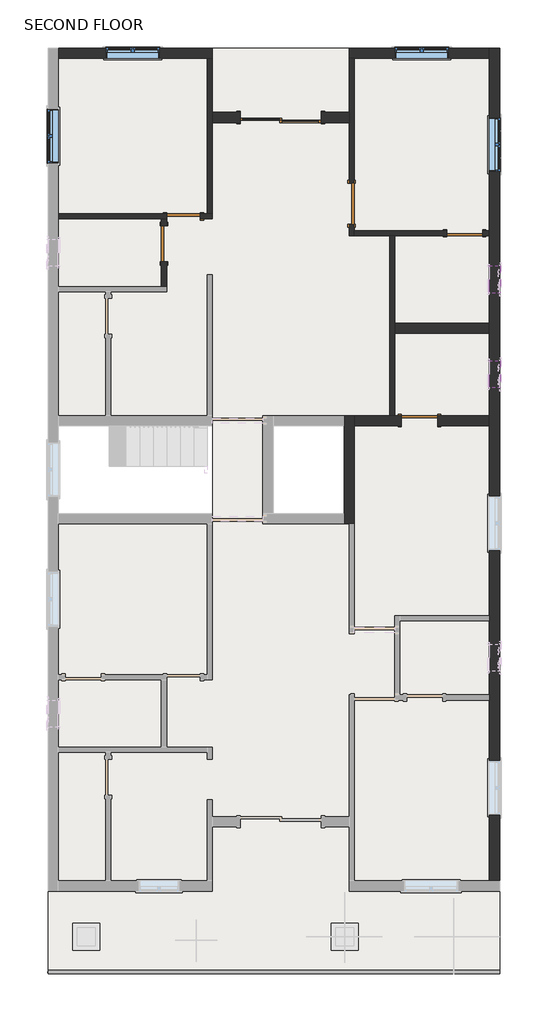
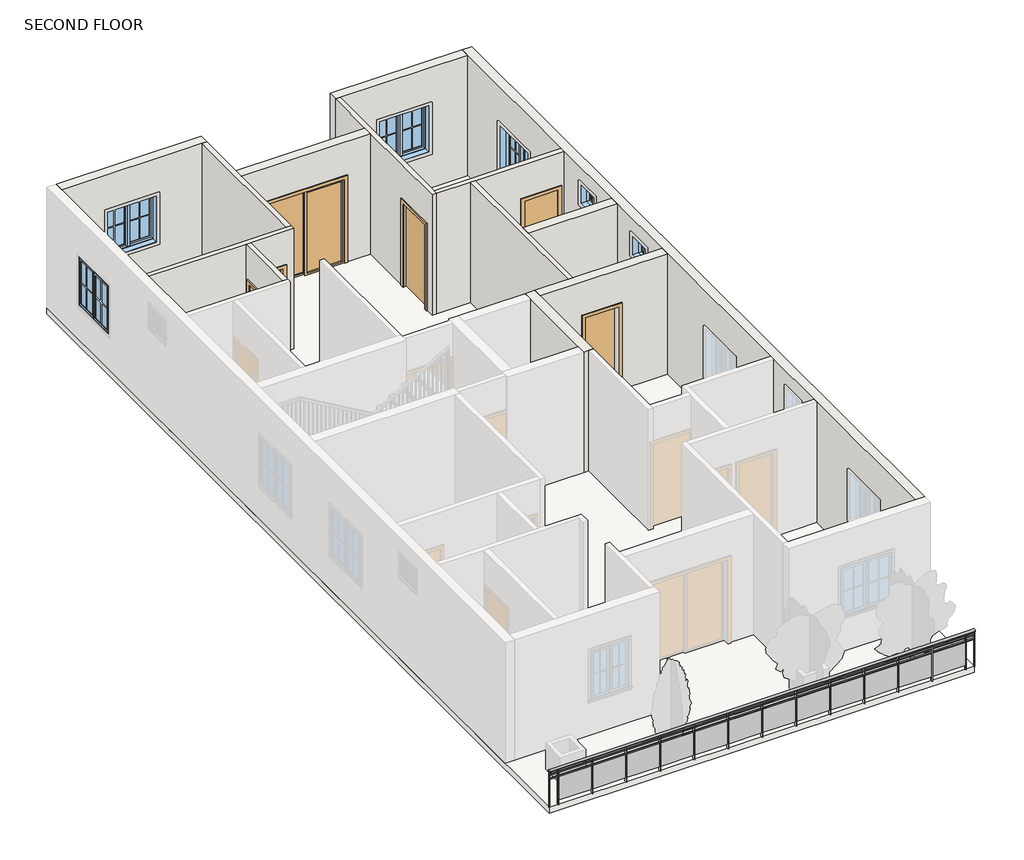
# One storey, part 2 of 4: 13 walls, 6 doors, 6 windows, 1 railing, 1 slab.
"""IFC4 building model written with IfcOpenShell, lengths in millimetres."""

from ifc_helpers import new_model, si_unit, point, frame, origin, place, context, project, spatial, polyline, ellipse_curve, trimmed, outline, extrude, faceted_brep, transform, mapped, element, save
from ifc_brep_helpers import plane_surface, extruded_surface, advanced_brep
from components import door_d4d75d1e, door_214872d5, door_d141acb4, door_38851409, door_7b345704, single_flush_3_x7_e5f9f3c4, window_79894727, window_casement_double_4_x4_af3140d2

model = new_model("IFC4")

# Units and contexts
model_context = context("Model", 3, world=origin())
ifc_project = project(units=[si_unit("LENGTHUNIT", "METRE", prefix="MILLI")], contexts=[model_context])

# Site, building, storey
site = spatial("IfcSite", under=ifc_project)
building = spatial("IfcBuilding", under=site)
storey = spatial("IfcBuildingStorey", under=building, Name="SECOND FLOOR", Elevation=6400.8)

# Doors
placement = place(None, origin())
door_shape = door_d4d75d1e(model_context)
element("IfcDoor", 1, ObjectType="Door-Double-Sliding : 72\" x 84\"", at=placement, inside=storey, context=model_context, shape_type="MappedRepresentation", body=[
    mapped(door_shape, transform((-1119.4789041, 8623.7153263, 6400.8), x_axis=(-1.0, 0.0, 0.0), y_axis=(0.0, -1.0, 0.0), z_axis=(0.0, 0.0, 1.0))),
])
door_2_shape = door_214872d5(model_context)
element("IfcDoor", 2, ObjectType="Single-Flush : 2'6\"X7'", at=placement, inside=storey, context=model_context, shape_type="MappedRepresentation", body=[
    mapped(door_2_shape, transform((-3310.2289041, 6267.8653263, 6400.8), x_axis=(1.0, 0.0, 0.0), y_axis=(0.0, 1.0, 0.0), z_axis=(0.0, 0.0, 1.0))),
])
door_3_shape = door_d141acb4(model_context)
element("IfcDoor", 3, ObjectType="Single-Flush : 2'8\"X7'", at=placement, inside=storey, context=model_context, shape_type="MappedRepresentation", body=[
    mapped(door_3_shape, transform((-3748.3789041, 5651.9153263, 6400.8), x_axis=(0.0, 1.0, 0.0), y_axis=(-1.0, 0.0, 0.0), z_axis=(0.0, 0.0, 1.0))),
])
door_4_shape = door_38851409(model_context)
element("IfcDoor", 4, ObjectType="Single-Flush : 2'8\"X7'", at=placement, inside=storey, context=model_context, shape_type="MappedRepresentation", body=[
    mapped(door_4_shape, transform((3027.0710959, 5886.8653263, 6400.8), x_axis=(1.0, 0.0, 0.0), y_axis=(0.0, 1.0, 0.0), z_axis=(0.0, 0.0, 1.0))),
])
door_5_shape = door_7b345704(model_context)
element("IfcDoor", 5, ObjectType="Single-Flush : 2'8\"X7'", at=placement, inside=storey, context=model_context, shape_type="MappedRepresentation", body=[
    mapped(door_5_shape, transform((2011.0710959, 1664.1153263, 6400.8), x_axis=(-1.0, 0.0, 0.0), y_axis=(0.0, -1.0, 0.0), z_axis=(0.0, 0.0, 1.0))),
])
single_flush_3_x7_shape = single_flush_3_x7_e5f9f3c4(model_context)
element("IfcDoor", 6, ObjectType="Single-Flush : 3'X7'", at=placement, inside=storey, context=model_context, shape_type="MappedRepresentation", body=[
    mapped(single_flush_3_x7_shape, transform((480.7210959, 6553.6153263, 6400.8), x_axis=(0.0, -1.0, 0.0), y_axis=(1.0, 0.0, 0.0), z_axis=(0.0, 0.0, 1.0))),
])

# Railing
element("IfcRailing", 7, ObjectType="Glass Panel - Bottom Fill", at=placement, inside=storey, context=model_context, shape_type="SolidModel", body=[
    advanced_brep(
    [(-6358.2289041, -10731.0846737, 7315.2), (-6358.2289041, -10807.2846737, 7315.2), (3814.4710959, -10731.0846737, 7315.2), (3814.4710959, -10807.2846737, 7315.2)],
    [
        (0, 1, ellipse_curve(frame((-6358.2289041, -10769.1846737, 7315.2), z_axis=(-1.0, 0.0, 0.0), x_axis=(0.0, -1.0, 0.0)), 38.1, 28.575)),
        (1, 0, ellipse_curve(frame((-6358.2289041, -10769.1846737, 7315.2), z_axis=(-1.0, 0.0, 0.0), x_axis=(0.0, -1.0, 0.0)), 38.1, 28.575)),
        (2, 3, ellipse_curve(frame((3814.4710959, -10769.1846737, 7315.2), z_axis=(1.0, 0.0, 0.0), x_axis=(0.0, -1.0, 0.0)), 38.1, 28.575)),
        (3, 2, ellipse_curve(frame((3814.4710959, -10769.1846737, 7315.2), z_axis=(1.0, 0.0, 0.0), x_axis=(0.0, -1.0, 0.0)), 38.1, 28.575)),
        (0, 2),
        (3, 1),
    ],
    [
        plane_surface(frame((-6358.2289041, -10769.1846737, 7315.2), z_axis=(-1.0, 0.0, 0.0), x_axis=(0.0, 1.0, 0.0))),
        plane_surface(frame((3814.4710959, -10769.1846737, 7315.2), z_axis=(1.0, 0.0, 0.0), x_axis=(0.0, 1.0, 0.0))),
        extruded_surface(trimmed(ellipse_curve(frame((3814.4710959, -10769.1846737, 7315.2), z_axis=(-1.0, 0.0, 0.0), x_axis=(0.0, -1.0, 0.0)), 38.1, 28.575), [point((3814.4710959, -10731.0846737, 7315.2))], [point((3814.4710959, -10807.2846737, 7315.2))], True, "CARTESIAN"), (-10172.7, 0.0, 0.0), 10172.7),
        extruded_surface(trimmed(ellipse_curve(frame((3814.4710959, -10769.1846737, 7315.2), z_axis=(-1.0, 0.0, 0.0), x_axis=(0.0, -1.0, 0.0)), 38.1, 28.575), [point((3814.4710959, -10807.2846737, 7315.2))], [point((3814.4710959, -10731.0846737, 7315.2))], True, "CARTESIAN"), (-10172.7, 0.0, 0.0), 10172.7),
    ],
    [
        (0, [[1, 2]]),
        (1, [[3, 4]]),
        (2, [[-1, 5, -4, 6]]),
        (3, [[-2, -6, -3, -5]]),
    ],
),
    extrude(outline(polyline([(-6358.2289041, -10781.8846737), (-6358.2289041, -10756.4846737), (3814.4710959, -10756.4846737), (3814.4710959, -10781.8846737), (-6358.2289041, -10781.8846737)])), frame((0.0, 0.0, 7200.9), z_axis=(0.0, 0.0, 1.0), x_axis=(1.0, 0.0, 0.0)), (0.0, 0.0, 1.0), 25.4),
    extrude(outline(polyline([(-6358.2289041, -10781.8846737), (-6358.2289041, -10756.4846737), (3814.4710959, -10756.4846737), (3814.4710959, -10781.8846737), (-6358.2289041, -10781.8846737)])), frame((0.0, 0.0, 7099.3), z_axis=(0.0, 0.0, 1.0), x_axis=(1.0, 0.0, 0.0)), (0.0, 0.0, 1.0), 25.4),
    extrude(outline(polyline([(3598.5710959, -10794.5846737), (3598.5710959, -10743.7846737), (3611.2710959, -10743.7846737), (3611.2710959, -10794.5846737), (3598.5710959, -10794.5846737)])), frame((0.0, 0.0, 6400.8), z_axis=(0.0, 0.0, 1.0), x_axis=(1.0, 0.0, 0.0)), (0.0, 0.0, 1.0), 885.825),
    extrude(outline(polyline([(2792.1210959, -10762.6495167), (3604.9210959, -10762.6495167), (3604.9210959, -10768.9995167), (2792.1210959, -10768.9995167), (2792.1210959, -10762.6495167)])), frame((0.0, 0.0, 6502.4), z_axis=(0.0, 0.0, 1.0), x_axis=(1.0, 0.0, 0.0)), (0.0, 0.0, 1.0), 596.9),
    extrude(outline(polyline([(2785.7710959, -10794.5846737), (2785.7710959, -10743.7846737), (2798.4710959, -10743.7846737), (2798.4710959, -10794.5846737), (2785.7710959, -10794.5846737)])), frame((0.0, 0.0, 6400.8), z_axis=(0.0, 0.0, 1.0), x_axis=(1.0, 0.0, 0.0)), (0.0, 0.0, 1.0), 885.825),
    extrude(outline(polyline([(1979.3210959, -10762.6495167), (2792.1210959, -10762.6495167), (2792.1210959, -10768.9995167), (1979.3210959, -10768.9995167), (1979.3210959, -10762.6495167)])), frame((0.0, 0.0, 6502.4), z_axis=(0.0, 0.0, 1.0), x_axis=(1.0, 0.0, 0.0)), (0.0, 0.0, 1.0), 596.9),
    extrude(outline(polyline([(1972.9710959, -10794.5846737), (1972.9710959, -10743.7846737), (1985.6710959, -10743.7846737), (1985.6710959, -10794.5846737), (1972.9710959, -10794.5846737)])), frame((0.0, 0.0, 6400.8), z_axis=(0.0, 0.0, 1.0), x_axis=(1.0, 0.0, 0.0)), (0.0, 0.0, 1.0), 885.825),
    extrude(outline(polyline([(1166.5210959, -10762.6495167), (1979.3210959, -10762.6495167), (1979.3210959, -10768.9995167), (1166.5210959, -10768.9995167), (1166.5210959, -10762.6495167)])), frame((0.0, 0.0, 6502.4), z_axis=(0.0, 0.0, 1.0), x_axis=(1.0, 0.0, 0.0)), (0.0, 0.0, 1.0), 596.9),
    extrude(outline(polyline([(1160.1710959, -10794.5846737), (1160.1710959, -10743.7846737), (1172.8710959, -10743.7846737), (1172.8710959, -10794.5846737), (1160.1710959, -10794.5846737)])), frame((0.0, 0.0, 6400.8), z_axis=(0.0, 0.0, 1.0), x_axis=(1.0, 0.0, 0.0)), (0.0, 0.0, 1.0), 885.825),
    extrude(outline(polyline([(353.7210959, -10762.6495167), (1166.5210959, -10762.6495167), (1166.5210959, -10768.9995167), (353.7210959, -10768.9995167), (353.7210959, -10762.6495167)])), frame((0.0, 0.0, 6502.4), z_axis=(0.0, 0.0, 1.0), x_axis=(1.0, 0.0, 0.0)), (0.0, 0.0, 1.0), 596.9),
    extrude(outline(polyline([(347.3710959, -10794.5846737), (347.3710959, -10743.7846737), (360.0710959, -10743.7846737), (360.0710959, -10794.5846737), (347.3710959, -10794.5846737)])), frame((0.0, 0.0, 6400.8), z_axis=(0.0, 0.0, 1.0), x_axis=(1.0, 0.0, 0.0)), (0.0, 0.0, 1.0), 885.825),
    extrude(outline(polyline([(-459.0789041, -10762.6495167), (353.7210959, -10762.6495167), (353.7210959, -10768.9995167), (-459.0789041, -10768.9995167), (-459.0789041, -10762.6495167)])), frame((0.0, 0.0, 6502.4), z_axis=(0.0, 0.0, 1.0), x_axis=(1.0, 0.0, 0.0)), (0.0, 0.0, 1.0), 596.9),
    extrude(outline(polyline([(-465.4289041, -10794.5846737), (-465.4289041, -10743.7846737), (-452.7289041, -10743.7846737), (-452.7289041, -10794.5846737), (-465.4289041, -10794.5846737)])), frame((0.0, 0.0, 6400.8), z_axis=(0.0, 0.0, 1.0), x_axis=(1.0, 0.0, 0.0)), (0.0, 0.0, 1.0), 885.825),
    extrude(outline(polyline([(-1271.8789041, -10762.6495167), (-459.0789041, -10762.6495167), (-459.0789041, -10768.9995167), (-1271.8789041, -10768.9995167), (-1271.8789041, -10762.6495167)])), frame((0.0, 0.0, 6502.4), z_axis=(0.0, 0.0, 1.0), x_axis=(1.0, 0.0, 0.0)), (0.0, 0.0, 1.0), 596.9),
    extrude(outline(polyline([(-1278.2289041, -10794.5846737), (-1278.2289041, -10743.7846737), (-1265.5289041, -10743.7846737), (-1265.5289041, -10794.5846737), (-1278.2289041, -10794.5846737)])), frame((0.0, 0.0, 6400.8), z_axis=(0.0, 0.0, 1.0), x_axis=(1.0, 0.0, 0.0)), (0.0, 0.0, 1.0), 885.825),
    extrude(outline(polyline([(-2084.6789041, -10762.6495167), (-1271.8789041, -10762.6495167), (-1271.8789041, -10768.9995167), (-2084.6789041, -10768.9995167), (-2084.6789041, -10762.6495167)])), frame((0.0, 0.0, 6502.4), z_axis=(0.0, 0.0, 1.0), x_axis=(1.0, 0.0, 0.0)), (0.0, 0.0, 1.0), 596.9),
    extrude(outline(polyline([(-2091.0289041, -10794.5846737), (-2091.0289041, -10743.7846737), (-2078.3289041, -10743.7846737), (-2078.3289041, -10794.5846737), (-2091.0289041, -10794.5846737)])), frame((0.0, 0.0, 6400.8), z_axis=(0.0, 0.0, 1.0), x_axis=(1.0, 0.0, 0.0)), (0.0, 0.0, 1.0), 885.825),
    extrude(outline(polyline([(-2897.4789041, -10762.6495167), (-2084.6789041, -10762.6495167), (-2084.6789041, -10768.9995167), (-2897.4789041, -10768.9995167), (-2897.4789041, -10762.6495167)])), frame((0.0, 0.0, 6502.4), z_axis=(0.0, 0.0, 1.0), x_axis=(1.0, 0.0, 0.0)), (0.0, 0.0, 1.0), 596.9),
    extrude(outline(polyline([(-2903.8289041, -10794.5846737), (-2903.8289041, -10743.7846737), (-2891.1289041, -10743.7846737), (-2891.1289041, -10794.5846737), (-2903.8289041, -10794.5846737)])), frame((0.0, 0.0, 6400.8), z_axis=(0.0, 0.0, 1.0), x_axis=(1.0, 0.0, 0.0)), (0.0, 0.0, 1.0), 885.825),
    extrude(outline(polyline([(-3710.2789041, -10762.6495167), (-2897.4789041, -10762.6495167), (-2897.4789041, -10768.9995167), (-3710.2789041, -10768.9995167), (-3710.2789041, -10762.6495167)])), frame((0.0, 0.0, 6502.4), z_axis=(0.0, 0.0, 1.0), x_axis=(1.0, 0.0, 0.0)), (0.0, 0.0, 1.0), 596.9),
    extrude(outline(polyline([(-3716.6289041, -10794.5846737), (-3716.6289041, -10743.7846737), (-3703.9289041, -10743.7846737), (-3703.9289041, -10794.5846737), (-3716.6289041, -10794.5846737)])), frame((0.0, 0.0, 6400.8), z_axis=(0.0, 0.0, 1.0), x_axis=(1.0, 0.0, 0.0)), (0.0, 0.0, 1.0), 885.825),
    extrude(outline(polyline([(-4523.0789041, -10762.6495167), (-3710.2789041, -10762.6495167), (-3710.2789041, -10768.9995167), (-4523.0789041, -10768.9995167), (-4523.0789041, -10762.6495167)])), frame((0.0, 0.0, 6502.4), z_axis=(0.0, 0.0, 1.0), x_axis=(1.0, 0.0, 0.0)), (0.0, 0.0, 1.0), 596.9),
    extrude(outline(polyline([(-4529.4289041, -10794.5846737), (-4529.4289041, -10743.7846737), (-4516.7289041, -10743.7846737), (-4516.7289041, -10794.5846737), (-4529.4289041, -10794.5846737)])), frame((0.0, 0.0, 6400.8), z_axis=(0.0, 0.0, 1.0), x_axis=(1.0, 0.0, 0.0)), (0.0, 0.0, 1.0), 885.825),
    extrude(outline(polyline([(-5335.8789041, -10762.6495167), (-4523.0789041, -10762.6495167), (-4523.0789041, -10768.9995167), (-5335.8789041, -10768.9995167), (-5335.8789041, -10762.6495167)])), frame((0.0, 0.0, 6502.4), z_axis=(0.0, 0.0, 1.0), x_axis=(1.0, 0.0, 0.0)), (0.0, 0.0, 1.0), 596.9),
    extrude(outline(polyline([(-5342.2289041, -10794.5846737), (-5342.2289041, -10743.7846737), (-5329.5289041, -10743.7846737), (-5329.5289041, -10794.5846737), (-5342.2289041, -10794.5846737)])), frame((0.0, 0.0, 6400.8), z_axis=(0.0, 0.0, 1.0), x_axis=(1.0, 0.0, 0.0)), (0.0, 0.0, 1.0), 885.825),
    extrude(outline(polyline([(-6148.6789041, -10762.6495167), (-5335.8789041, -10762.6495167), (-5335.8789041, -10768.9995167), (-6148.6789041, -10768.9995167), (-6148.6789041, -10762.6495167)])), frame((0.0, 0.0, 6502.4), z_axis=(0.0, 0.0, 1.0), x_axis=(1.0, 0.0, 0.0)), (0.0, 0.0, 1.0), 596.9),
    extrude(outline(polyline([(-6155.0289041, -10794.5846737), (-6155.0289041, -10743.7846737), (-6142.3289041, -10743.7846737), (-6142.3289041, -10794.5846737), (-6155.0289041, -10794.5846737)])), frame((0.0, 0.0, 6400.8), z_axis=(0.0, 0.0, 1.0), x_axis=(1.0, 0.0, 0.0)), (0.0, 0.0, 1.0), 885.825),
    extrude(outline(polyline([(3801.7710959, -10778.7096737), (3801.7710959, -10759.6596737), (3820.8210959, -10759.6596737), (3820.8210959, -10778.7096737), (3801.7710959, -10778.7096737)])), frame((0.0, 0.0, 6400.8), z_axis=(0.0, 0.0, 1.0), x_axis=(1.0, 0.0, 0.0)), (0.0, 0.0, 1.0), 885.825),
    extrude(outline(polyline([(-6364.5789041, -10778.7096737), (-6364.5789041, -10759.6596737), (-6345.5289041, -10759.6596737), (-6345.5289041, -10778.7096737), (-6364.5789041, -10778.7096737)])), frame((0.0, 0.0, 6400.8), z_axis=(0.0, 0.0, 1.0), x_axis=(1.0, 0.0, 0.0)), (0.0, 0.0, 1.0), 885.825),
])

# Slab
element("IfcSlab", 8, ObjectType="6\"", at=placement, inside=storey, context=model_context, shape_type="SweptSolid", body=[
    extrude(outline(polyline([(3814.4710959, 10058.8153263), (3814.4710959, -10769.1846737), (-6358.2289041, -10769.1846737), (-6358.2289041, 10058.8153263), (3814.4710959, 10058.8153263)]), holes=[polyline([(-2662.5289041, 1549.8153263), (-6129.6289041, 1549.8153263), (-6129.6289041, -431.3846737), (-2662.5289041, -431.3846737), (-2662.5289041, 1549.8153263)]), polyline([(537.8710959, 1778.4153263), (-1519.5289041, 1778.4153263), (-1519.5289041, -659.9846737), (537.8710959, -659.9846737), (537.8710959, 1778.4153263)])]), frame((0.0, 0.0, 6248.4), z_axis=(0.0, 0.0, 1.0), x_axis=(1.0, 0.0, 0.0)), (0.0, 0.0, 1.0), 152.4),
])

# Walls
element("IfcWall", 9, ObjectType="4.5\"", at=placement, inside=storey, context=model_context, shape_type="SweptSolid", body=[
    extrude(outline(polyline([(6210.7153263, 6400.8), (6058.3153263, 6400.8), (6058.3153263, 8534.4), (5245.5153263, 8534.4), (5245.5153263, 6400.8), (4686.7153263, 6400.8), (4686.7153263, 9448.8), (6210.7153263, 9448.8), (6210.7153263, 6400.8)])), frame((-3805.5289041, 0.0, 0.0), z_axis=(1.0, 0.0, 0.0), x_axis=(0.0, 1.0, 0.0)), (0.0, 0.0, 1.0), 114.3),
])
element("IfcWall", 10, ObjectType="4.5\"", at=placement, inside=storey, context=model_context, shape_type="Brep", body=[
    faceted_brep([(-2929.2289041, 6210.7153263, 8534.4), (-2929.2289041, 6210.7153263, 6400.8), (-2662.5289041, 6210.7153263, 6400.8), (-2662.5289041, 6210.7153263, 9448.8), (-3691.2289041, 6210.7153263, 9448.8), (-3805.5289041, 6210.7153263, 9448.8), (-6129.6289041, 6210.7153263, 9448.8), (-6129.6289041, 6210.7153263, 6400.8), (-3805.5289041, 6210.7153263, 6400.8), (-3691.2289041, 6210.7153263, 6400.8), (-3691.2289041, 6210.7153263, 8534.4), (-2662.5289041, 6325.0153263, 6400.8), (-2776.8289041, 6325.0153263, 6400.8), (-2929.2289041, 6325.0153263, 6400.8), (-2929.2289041, 6325.0153263, 8534.4), (-3691.2289041, 6325.0153263, 8534.4), (-3691.2289041, 6325.0153263, 6400.8), (-6129.6289041, 6325.0153263, 6400.8), (-6129.6289041, 6325.0153263, 9448.8), (-2776.8289041, 6325.0153263, 9448.8), (-2662.5289041, 6325.0153263, 9448.8)], [[[0, 1, 2, 3, 4, 5, 6, 7, 8, 9, 10]], [[11, 12, 13, 14, 15, 16, 17, 18, 19, 20]], [[2, 1, 13, 12, 11]], [[9, 8, 7, 17, 16]], [[6, 5, 4, 3, 20, 19, 18]], [[7, 6, 18, 17]], [[3, 2, 11, 20]], [[14, 13, 1, 0]], [[15, 14, 0, 10]], [[16, 15, 10, 9]]]),
])
element("IfcWall", 11, ObjectType="4.5\"", at=placement, inside=storey, context=model_context, shape_type="Brep", body=[
    faceted_brep([(-2662.5289041, 6325.0153263, 6400.8), (-2662.5289041, 8382.4153263, 6400.8), (-2662.5289041, 8611.0153263, 6400.8), (-2662.5289041, 9830.2153263, 6400.8), (-2662.5289041, 9830.2153263, 9448.8), (-2662.5289041, 8611.0153263, 9448.8), (-2662.5289041, 8382.4153263, 9448.8), (-2662.5289041, 6325.0153263, 9448.8), (-2776.8289041, 6325.0153263, 6400.8), (-2776.8289041, 6325.0153263, 9448.8), (-2776.8289041, 9830.2153263, 9448.8), (-2776.8289041, 9830.2153263, 6400.8)], [[[0, 1, 2, 3, 4, 5, 6, 7]], [[8, 9, 10, 11]], [[3, 2, 1, 0, 8, 11]], [[7, 6, 5, 4, 10, 9]], [[0, 7, 9, 8]], [[4, 3, 11, 10]]]),
])
element("IfcWall", 12, ObjectType="4.5\"", at=placement, inside=storey, context=model_context, shape_type="Brep", body=[
    faceted_brep([(423.5710959, 6096.4153263, 8534.4), (423.5710959, 6096.4153263, 6400.8), (423.5710959, 5829.7153263, 6400.8), (423.5710959, 5829.7153263, 9448.8), (423.5710959, 8382.4153263, 9448.8), (423.5710959, 8611.0153263, 9448.8), (423.5710959, 9830.2153263, 9448.8), (423.5710959, 9830.2153263, 6400.8), (423.5710959, 8611.0153263, 6400.8), (423.5710959, 8382.4153263, 6400.8), (423.5710959, 7010.8153263, 6400.8), (423.5710959, 7010.8153263, 8534.4), (537.8710959, 5829.7153263, 6400.8), (537.8710959, 5944.0153263, 6400.8), (537.8710959, 6096.4153263, 6400.8), (537.8710959, 6096.4153263, 8534.4), (537.8710959, 7010.8153263, 8534.4), (537.8710959, 7010.8153263, 6400.8), (537.8710959, 9830.2153263, 6400.8), (537.8710959, 9830.2153263, 9448.8), (537.8710959, 5944.0153263, 9448.8), (537.8710959, 5829.7153263, 9448.8)], [[[0, 1, 2, 3, 4, 5, 6, 7, 8, 9, 10, 11]], [[12, 13, 14, 15, 16, 17, 18, 19, 20, 21]], [[2, 1, 14, 13, 12]], [[10, 9, 8, 7, 18, 17]], [[6, 5, 4, 3, 21, 20, 19]], [[7, 6, 19, 18]], [[3, 2, 12, 21]], [[15, 14, 1, 0]], [[16, 15, 0, 11]], [[17, 16, 11, 10]]]),
])
element("IfcWall", 13, ObjectType="4.5\"", at=placement, inside=storey, context=model_context, shape_type="Brep", body=[
    faceted_brep([(3433.4710959, 5829.7153263, 8534.4), (3433.4710959, 5829.7153263, 6400.8), (3585.8710959, 5829.7153263, 6400.8), (3585.8710959, 5829.7153263, 9448.8), (1452.2710959, 5829.7153263, 9448.8), (1337.9710959, 5829.7153263, 9448.8), (537.8710959, 5829.7153263, 9448.8), (537.8710959, 5829.7153263, 6400.8), (1337.9710959, 5829.7153263, 6400.8), (1452.2710959, 5829.7153263, 6400.8), (2620.6710959, 5829.7153263, 6400.8), (2620.6710959, 5829.7153263, 8534.4), (3585.8710959, 5944.0153263, 6400.8), (3433.4710959, 5944.0153263, 6400.8), (3433.4710959, 5944.0153263, 8534.4), (2620.6710959, 5944.0153263, 8534.4), (2620.6710959, 5944.0153263, 6400.8), (537.8710959, 5944.0153263, 6400.8), (537.8710959, 5944.0153263, 9448.8), (3585.8710959, 5944.0153263, 9448.8)], [[[0, 1, 2, 3, 4, 5, 6, 7, 8, 9, 10, 11]], [[12, 13, 14, 15, 16, 17, 18, 19]], [[2, 1, 13, 12]], [[10, 9, 8, 7, 17, 16]], [[6, 5, 4, 3, 19, 18]], [[7, 6, 18, 17]], [[3, 2, 12, 19]], [[14, 13, 1, 0]], [[15, 14, 0, 11]], [[16, 15, 11, 10]]]),
])
element("IfcWall", 14, ObjectType="4.5\"", at=placement, inside=storey, context=model_context, shape_type="Brep", body=[
    faceted_brep([(1337.9710959, 5829.7153263, 6400.8), (1337.9710959, 1778.4153263, 6400.8), (1337.9710959, 1778.4153263, 9448.8), (1337.9710959, 5829.7153263, 9448.8), (1452.2710959, 5829.7153263, 6400.8), (1452.2710959, 5829.7153263, 9448.8), (1452.2710959, 3861.2153263, 9448.8), (1452.2710959, 3632.6153263, 9448.8), (1452.2710959, 1778.4153263, 9448.8), (1452.2710959, 1778.4153263, 6400.8), (1452.2710959, 3632.6153263, 6400.8), (1452.2710959, 3861.2153263, 6400.8)], [[[0, 1, 2, 3]], [[4, 5, 6, 7, 8, 9, 10, 11]], [[1, 0, 4, 11, 10, 9]], [[3, 2, 8, 7, 6, 5]], [[2, 1, 9, 8]], [[0, 3, 5, 4]]]),
])
element("IfcWall", 15, ObjectType="9\"", at=placement, inside=storey, context=model_context, shape_type="Brep", body=[
    faceted_brep([(3814.4710959, -8711.7846737, 6400.8), (3814.4710959, 10058.8153263, 6400.8), (3814.4710959, 10058.8153263, 9448.8), (3814.4710959, -8711.7846737, 9448.8), (3814.4710959, -7225.8846737, 8534.4), (3814.4710959, -6006.6846737, 8534.4), (3814.4710959, -6006.6846737, 7315.2), (3814.4710959, -7225.8846737, 7315.2), (3814.4710959, -1256.8846737, 8534.4), (3814.4710959, -37.6846737, 8534.4), (3814.4710959, -37.6846737, 7315.2), (3814.4710959, -1256.8846737, 7315.2), (3814.4710959, 7277.5153263, 8534.4), (3814.4710959, 8496.7153263, 8534.4), (3814.4710959, 8496.7153263, 7315.2), (3814.4710959, 7277.5153263, 7315.2), (3814.4710959, -3987.3846737, 9067.8), (3814.4710959, -3377.7846737, 9067.8), (3814.4710959, -3377.7846737, 8534.4), (3814.4710959, -3987.3846737, 8534.4), (3814.4710959, 2400.7153263, 9067.8), (3814.4710959, 3010.3153263, 9067.8), (3814.4710959, 3010.3153263, 8534.4), (3814.4710959, 2400.7153263, 8534.4), (3814.4710959, 4540.6653263, 9067.8), (3814.4710959, 5150.2653263, 9067.8), (3814.4710959, 5150.2653263, 8534.4), (3814.4710959, 4540.6653263, 8534.4), (3585.8710959, -8711.7846737, 6400.8), (3585.8710959, -8711.7846737, 9448.8), (3585.8710959, -4635.0846737, 9448.8), (3585.8710959, -4520.7846737, 9448.8), (3585.8710959, -2844.3846737, 9448.8), (3585.8710959, -2730.0846737, 9448.8), (3585.8710959, 1549.8153263, 9448.8), (3585.8710959, 1778.4153263, 9448.8), (3585.8710959, 3632.6153263, 9448.8), (3585.8710959, 3861.2153263, 9448.8), (3585.8710959, 5829.7153263, 9448.8), (3585.8710959, 5944.0153263, 9448.8), (3585.8710959, 9830.2153263, 9448.8), (3585.8710959, 10058.8153263, 9448.8), (3585.8710959, 10058.8153263, 6400.8), (3585.8710959, 9830.2153263, 6400.8), (3585.8710959, 5944.0153263, 6400.8), (3585.8710959, 5829.7153263, 6400.8), (3585.8710959, 3861.2153263, 6400.8), (3585.8710959, 3632.6153263, 6400.8), (3585.8710959, 1778.4153263, 6400.8), (3585.8710959, 1549.8153263, 6400.8), (3585.8710959, -2730.0846737, 6400.8), (3585.8710959, -2844.3846737, 6400.8), (3585.8710959, -4520.7846737, 6400.8), (3585.8710959, -4635.0846737, 6400.8), (3585.8710959, -7225.8846737, 8534.4), (3585.8710959, -7225.8846737, 7315.2), (3585.8710959, -6006.6846737, 7315.2), (3585.8710959, -6006.6846737, 8534.4), (3585.8710959, -1256.8846737, 8534.4), (3585.8710959, -1256.8846737, 7315.2), (3585.8710959, -37.6846737, 7315.2), (3585.8710959, -37.6846737, 8534.4), (3585.8710959, 7277.5153263, 8534.4), (3585.8710959, 7277.5153263, 7315.2), (3585.8710959, 8496.7153263, 7315.2), (3585.8710959, 8496.7153263, 8534.4), (3585.8710959, -3987.3846737, 9067.8), (3585.8710959, -3987.3846737, 8534.4), (3585.8710959, -3377.7846737, 8534.4), (3585.8710959, -3377.7846737, 9067.8), (3585.8710959, 2400.7153263, 9067.8), (3585.8710959, 2400.7153263, 8534.4), (3585.8710959, 3010.3153263, 8534.4), (3585.8710959, 3010.3153263, 9067.8), (3585.8710959, 4540.6653263, 9067.8), (3585.8710959, 4540.6653263, 8534.4), (3585.8710959, 5150.2653263, 8534.4), (3585.8710959, 5150.2653263, 9067.8)], [[[0, 1, 2, 3], [4, 5, 6, 7], [8, 9, 10, 11], [12, 13, 14, 15], [16, 17, 18, 19], [20, 21, 22, 23], [24, 25, 26, 27]], [[28, 29, 30, 31, 32, 33, 34, 35, 36, 37, 38, 39, 40, 41, 42, 43, 44, 45, 46, 47, 48, 49, 50, 51, 52, 53], [54, 55, 56, 57], [58, 59, 60, 61], [62, 63, 64, 65], [66, 67, 68, 69], [70, 71, 72, 73], [74, 75, 76, 77]], [[1, 0, 28, 53, 52, 51, 50, 49, 48, 47, 46, 45, 44, 43, 42]], [[3, 2, 41, 40, 39, 38, 37, 36, 35, 34, 33, 32, 31, 30, 29]], [[0, 3, 29, 28]], [[2, 1, 42, 41]], [[55, 54, 4, 7]], [[56, 55, 7, 6]], [[57, 56, 6, 5]], [[54, 57, 5, 4]], [[59, 58, 8, 11]], [[60, 59, 11, 10]], [[61, 60, 10, 9]], [[58, 61, 9, 8]], [[63, 62, 12, 15]], [[64, 63, 15, 14]], [[65, 64, 14, 13]], [[62, 65, 13, 12]], [[67, 66, 16, 19]], [[68, 67, 19, 18]], [[69, 68, 18, 17]], [[66, 69, 17, 16]], [[71, 70, 20, 23]], [[72, 71, 23, 22]], [[73, 72, 22, 21]], [[70, 73, 21, 20]], [[75, 74, 24, 27]], [[76, 75, 27, 26]], [[77, 76, 26, 25]], [[74, 77, 25, 24]]]),
])
element("IfcWall", 16, ObjectType="9\"", at=placement, inside=storey, context=model_context, shape_type="Brep", body=[
    faceted_brep([(3585.8710959, 10058.8153263, 6400.8), (423.5710959, 10058.8153263, 6400.8), (423.5710959, 10058.8153263, 9448.8), (3585.8710959, 10058.8153263, 9448.8), (2671.4710959, 10058.8153263, 8534.4), (1452.2710959, 10058.8153263, 8534.4), (1452.2710959, 10058.8153263, 7315.2), (2671.4710959, 10058.8153263, 7315.2), (3585.8710959, 9830.2153263, 6400.8), (3585.8710959, 9830.2153263, 9448.8), (537.8710959, 9830.2153263, 9448.8), (423.5710959, 9830.2153263, 9448.8), (423.5710959, 9830.2153263, 6400.8), (537.8710959, 9830.2153263, 6400.8), (2671.4710959, 9830.2153263, 8534.4), (2671.4710959, 9830.2153263, 7315.2), (1452.2710959, 9830.2153263, 7315.2), (1452.2710959, 9830.2153263, 8534.4)], [[[0, 1, 2, 3], [4, 5, 6, 7]], [[8, 9, 10, 11, 12, 13], [14, 15, 16, 17]], [[1, 0, 8, 13, 12]], [[3, 2, 11, 10, 9]], [[0, 3, 9, 8]], [[2, 1, 12, 11]], [[15, 14, 4, 7]], [[16, 15, 7, 6]], [[17, 16, 6, 5]], [[14, 17, 5, 4]]]),
])
element("IfcWall", 17, ObjectType="9\"", at=placement, inside=storey, context=model_context, shape_type="Brep", body=[
    faceted_brep([(-2662.5289041, 10058.8153263, 6400.8), (-6129.6289041, 10058.8153263, 6400.8), (-6129.6289041, 10058.8153263, 9448.8), (-2662.5289041, 10058.8153263, 9448.8), (-3843.6289041, 10058.8153263, 8534.4), (-5062.8289041, 10058.8153263, 8534.4), (-5062.8289041, 10058.8153263, 7315.2), (-3843.6289041, 10058.8153263, 7315.2), (-2662.5289041, 9830.2153263, 6400.8), (-2662.5289041, 9830.2153263, 9448.8), (-2776.8289041, 9830.2153263, 9448.8), (-6129.6289041, 9830.2153263, 9448.8), (-6129.6289041, 9830.2153263, 6400.8), (-2776.8289041, 9830.2153263, 6400.8), (-3843.6289041, 9830.2153263, 8534.4), (-3843.6289041, 9830.2153263, 7315.2), (-5062.8289041, 9830.2153263, 7315.2), (-5062.8289041, 9830.2153263, 8534.4)], [[[0, 1, 2, 3], [4, 5, 6, 7]], [[8, 9, 10, 11, 12, 13], [14, 15, 16, 17]], [[1, 0, 8, 13, 12]], [[3, 2, 11, 10, 9]], [[2, 1, 12, 11]], [[0, 3, 9, 8]], [[15, 14, 4, 7]], [[16, 15, 7, 6]], [[17, 16, 6, 5]], [[14, 17, 5, 4]]]),
])
element("IfcWall", 18, ObjectType="9\"", at=placement, inside=storey, context=model_context, shape_type="Brep", body=[
    faceted_brep([(309.2710959, 1778.4153263, 6400.8), (309.2710959, 1549.8153263, 6400.8), (309.2710959, -431.3846737, 6400.8), (309.2710959, -659.9846737, 6400.8), (309.2710959, -659.9846737, 9448.8), (309.2710959, -431.3846737, 9448.8), (309.2710959, 1549.8153263, 9448.8), (309.2710959, 1778.4153263, 9448.8), (537.8710959, 1778.4153263, 6400.8), (537.8710959, 1778.4153263, 9448.8), (537.8710959, 1549.8153263, 9448.8), (537.8710959, -659.9846737, 9448.8), (537.8710959, -659.9846737, 6400.8), (537.8710959, 1549.8153263, 6400.8), (423.5710959, -659.9846737, 6400.8), (423.5710959, -659.9846737, 9448.8)], [[[0, 1, 2, 3, 4, 5, 6, 7]], [[8, 9, 10, 11, 12, 13]], [[3, 2, 1, 0, 8, 13, 12, 14]], [[7, 6, 5, 4, 15, 11, 10, 9]], [[4, 3, 14, 12, 11, 15]], [[0, 7, 9, 8]]]),
])
element("IfcWall", 19, ObjectType="9\"", at=placement, inside=storey, context=model_context, shape_type="Brep", body=[
    faceted_brep([(537.8710959, 1549.8153263, 6400.8), (1604.6710959, 1549.8153263, 6400.8), (1604.6710959, 1549.8153263, 8534.4), (2417.4710959, 1549.8153263, 8534.4), (2417.4710959, 1549.8153263, 6400.8), (3585.8710959, 1549.8153263, 6400.8), (3585.8710959, 1549.8153263, 9448.8), (537.8710959, 1549.8153263, 9448.8), (1604.6710959, 1778.4153263, 8534.4), (1604.6710959, 1778.4153263, 6400.8), (1452.2710959, 1778.4153263, 6400.8), (1337.9710959, 1778.4153263, 6400.8), (537.8710959, 1778.4153263, 6400.8), (537.8710959, 1778.4153263, 9448.8), (1337.9710959, 1778.4153263, 9448.8), (1452.2710959, 1778.4153263, 9448.8), (3585.8710959, 1778.4153263, 9448.8), (3585.8710959, 1778.4153263, 6400.8), (2417.4710959, 1778.4153263, 6400.8), (2417.4710959, 1778.4153263, 8534.4)], [[[0, 1, 2, 3, 4, 5, 6, 7]], [[8, 9, 10, 11, 12, 13, 14, 15, 16, 17, 18, 19]], [[18, 17, 5, 4]], [[12, 11, 10, 9, 1, 0]], [[7, 6, 16, 15, 14, 13]], [[0, 7, 13, 12]], [[6, 5, 17, 16]], [[2, 1, 9, 8]], [[3, 2, 8, 19]], [[4, 3, 19, 18]]]),
])
element("IfcWall", 20, ObjectType="9\"", at=placement, inside=storey, context=model_context, shape_type="SweptSolid", body=[
    extrude(outline(polyline([(1452.2710959, 3861.2153263), (3585.8710959, 3861.2153263), (3585.8710959, 3632.6153263), (1452.2710959, 3632.6153263), (1452.2710959, 3861.2153263)])), frame((0.0, 0.0, 6400.8), z_axis=(0.0, 0.0, 1.0), x_axis=(1.0, 0.0, 0.0)), (0.0, 0.0, 1.0), 3048.0),
])
element("IfcWall", 21, ObjectType="9\"", at=placement, inside=storey, context=model_context, shape_type="SweptSolid", body=[
    extrude(outline(polyline([(6400.8, -2662.5289041), (6400.8, -2033.8789041), (8534.4, -2033.8789041), (8534.4, -205.0789041), (6400.8, -205.0789041), (6400.8, 423.5710959), (9448.8, 423.5710959), (9448.8, -2662.5289041), (6400.8, -2662.5289041)])), frame((0.0, 8382.4153263, 0.0), z_axis=(0.0, 1.0, 0.0), x_axis=(0.0, 0.0, 1.0)), (0.0, 0.0, 1.0), 228.6),
])

# Windows
window_shape = window_79894727(model_context)
element("IfcWindow", 22, ObjectType="Window-Casement-Double : 2'X1'9\"", at=placement, inside=storey, context=model_context, shape_type="MappedRepresentation", body=[
    mapped(window_shape, transform((3700.1710959, 2705.5153263, 6400.8), x_axis=(0.0, -1.0, 0.0), y_axis=(1.0, 0.0, 0.0), z_axis=(0.0, 0.0, 1.0))),
])
element("IfcWindow", 23, ObjectType="Window-Casement-Double : 2'X1'9\"", at=placement, inside=storey, context=model_context, shape_type="MappedRepresentation", body=[
    mapped(window_shape, transform((3700.1710959, 4845.4653263, 6400.8), x_axis=(0.0, -1.0, 0.0), y_axis=(1.0, 0.0, 0.0), z_axis=(0.0, 0.0, 1.0))),
])
window_casement_double_4_x4_shape = window_casement_double_4_x4_af3140d2(model_context)
element("IfcWindow", 24, ObjectType="Window-Casement-Double : 4'X4'", at=placement, inside=storey, context=model_context, shape_type="MappedRepresentation", body=[
    mapped(window_casement_double_4_x4_shape, transform((-4453.2289041, 9944.5153263, 6400.8), x_axis=(1.0, 0.0, 0.0), y_axis=(0.0, 1.0, 0.0), z_axis=(0.0, 0.0, 1.0))),
])
element("IfcWindow", 25, ObjectType="Window-Casement-Double : 4'X4'", at=placement, inside=storey, context=model_context, shape_type="MappedRepresentation", body=[
    mapped(window_casement_double_4_x4_shape, transform((-6243.9289041, 8077.6153263, 6400.8), x_axis=(0.0, 1.0, 0.0), y_axis=(-1.0, 0.0, 0.0), z_axis=(0.0, 0.0, 1.0))),
])
element("IfcWindow", 26, ObjectType="Window-Casement-Double : 4'X4'", at=placement, inside=storey, context=model_context, shape_type="MappedRepresentation", body=[
    mapped(window_casement_double_4_x4_shape, transform((3700.1710959, 7887.1153263, 6400.8), x_axis=(0.0, -1.0, 0.0), y_axis=(1.0, 0.0, 0.0), z_axis=(0.0, 0.0, 1.0))),
])
element("IfcWindow", 27, ObjectType="Window-Casement-Double : 4'X4'", at=placement, inside=storey, context=model_context, shape_type="MappedRepresentation", body=[
    mapped(window_casement_double_4_x4_shape, transform((2061.8710959, 9944.5153263, 6400.8), x_axis=(1.0, 0.0, 0.0), y_axis=(0.0, 1.0, 0.0), z_axis=(0.0, 0.0, 1.0))),
])

save(model, "model.ifc")

# Revit data of these elements
# Type "Door-Double-Sliding : 72\" x 84\""
#   Type Mark = "14"
#   Construction Type Id = "opn-d45"
#   Assembly Code = "C1020"
#   Analytic Construction = "Wood frame, double glass door "
#   Thickness = 0' - 2"
#   Thermal Resistance (R) = 1.8150 (h·ft²·°F)/BTU
#   Heat Transfer Coefficient (U) = 0.5510 BTU/(h·ft²·°F)
#   Height = 7' - 0"
#   Rail Width = 0' - 2"
#   Stiles = 0' - 2"
#   Trim Projection Ext = 0' - 1"
#   Trim Projection Int = 0' - 1"
#   Trim Width = 0' - 3"
#   Width = 6' - 0"
#   Define Thermal Properties by = 1
#   Glazing = Glass
#   Panel Material = Wood - Birch - Solid Stained Light Low Gloss
#   Trim Material = Paint - Sienna
#   Visual Light Transmittance = 0
#   Solar Heat Gain Coefficient = 0
#   Function = (empty or 0)
#   Wall Closure = (empty or 0)
# Type "Single-Flush : 2'6\"X7'"
#   Type Mark = "13"
#   Construction Type Id = "MDOOR"
#   Assembly Code = "C1020"
#   Analytic Construction = "Metal"
#   Thickness = 0' - 2"
#   Heat Transfer Coefficient (U) = 0.651978 BTU/(h·ft²·°F)
#   Height = 7' - 0"
#   Trim Projection Ext = 0' - 1"
#   Trim Projection Int = 0' - 1"
#   Trim Width = 0' - 3"
#   Width = 2' - 6"
#   Define Thermal Properties by = 1
#   Door Material = Door - Panel
#   Frame Material = Door - Frame
#   Visual Light Transmittance = 0
#   Solar Heat Gain Coefficient = 0
#   Function = (empty or 0)
#   Wall Closure = (empty or 0)
# Type "Single-Flush : 2'8\"X7'"
#   Type Mark = "12"
#   Construction Type Id = "MDOOR"
#   Assembly Code = "C1020"
#   Analytic Construction = "Metal"
#   Thickness = 0' - 2"
#   Heat Transfer Coefficient (U) = 0.651978 BTU/(h·ft²·°F)
#   Height = 7' - 0"
#   Trim Projection Ext = 0' - 1"
#   Trim Projection Int = 0' - 1"
#   Trim Width = 0' - 3"
#   Width = 2' - 8"
#   Define Thermal Properties by = 1
#   Door Material = Door - Panel
#   Frame Material = Door - Frame
#   Visual Light Transmittance = 0
#   Solar Heat Gain Coefficient = 0
#   Function = (empty or 0)
#   Wall Closure = (empty or 0)
# Type "Single-Flush : 3'X7'"
#   Type Mark = "8"
#   Construction Type Id = "MDOOR"
#   Assembly Code = "C1020"
#   Analytic Construction = "Metal"
#   Thickness = 0' - 2"
#   Heat Transfer Coefficient (U) = 0.651978 BTU/(h·ft²·°F)
#   Height = 7' - 0"
#   Trim Projection Ext = 0' - 1"
#   Trim Projection Int = 0' - 1"
#   Trim Width = 0' - 3"
#   Width = 3' - 0"
#   Define Thermal Properties by = 1
#   Door Material = Door - Panel
#   Frame Material = Door - Frame
#   Visual Light Transmittance = 0
#   Solar Heat Gain Coefficient = 0
#   Function = (empty or 0)
#   Wall Closure = (empty or 0)
# Type "Glass Panel - Bottom Fill"
#   Assembly Code = "C2010400"
#   built-in parameter 1008612 = 0.0416667 (stored number, unit not read)
#   built-in parameter 1008611 = 0.0416667 (stored number, unit not read)
#   built-in parameter 1008609 = 0.333333 (stored number, unit not read)
#   built-in parameter 1008604 = 0.166667 (stored number, unit not read)
#   built-in parameter 1008603 = 0.166667 (stored number, unit not read)
#   Railing Height = 3' - 0"
#   built-in parameter 1008630 = 2
#   built-in parameter 1008610 = 2
#   built-in parameter 1008618 = Baluster - Square : 3/4"
# Type "6\""
#   Assembly Code = "B1010"
#   Function = 0
#   Layers, outside or top first: 0' - 6" no material (function 1)
# Type "4.5\""
#   Assembly Code = "B2010"
#   Layers, outside or top first: 0' - 4 1/2" no material (function 1)
# Type "9\""
#   Assembly Code = "B2010"
#   Layers, outside or top first: 0' - 9" "WALL" (function 1)
# Type "Window-Casement-Double : 2'X1'9\""
#   Type Mark = "22"
#   Fire Rating = "0.5h"
#   Assembly Code = "B2020100"
#   Analytic Construction = "Double glazing - domestic"
#   Frame Extension [instance default] = 0' - 0 1/4"
#   Window Inset [instance default] = 0' - 0"
#   Wall Thickness [instance default] = 0' - 6"
#   Interior Wall Closure [instance default] = 0' - 2 1/4"
#   Half Width = 1' - 0"
#   Visual Light Transmittance = 0.81
#   Thermal Resistance (R) = 1.8146 (h·ft²·°F)/BTU
#   Solar Heat Gain Coefficient = 0.76
#   Rough Width = 2' - 0 1/2"
#   Rough Height = 1' - 9 1/2"
#   Height = 1' - 9"
#   Heat Transfer Coefficient (U) = 0.5511 BTU/(h·ft²·°F)
#   Exterior Wall Closure [instance default] = 0' - 1 1/4"
#   Extension Jamb [instance default] = 0' - 2 1/4"
#   Default Sill Height = 7' - 0"
#   Width = 2' - 0"
#   Muntin Visibility = yes
#   Interior Trim Visibility [instance default] = yes
#   Exterior Trim Visibility [instance default] = yes
#   Extension Jamb Visibility [instance default] = yes
#   Interior Trim Material = Wood - Stained
#   Muntin Pattern = Muntin Pattern_2x2 : Muntin Pattern_2x2
#   Interior Trim = Trim-Window-Interior-Flat : Picture Frame
#   Interior Frame Material = Wood - Stained
#   Glass Panel Material = Glass
#   Exterior Trim Material = Clad - White
#   Exterior Trim = Trim-Window-Exterior-Flat : with Sill
#   Exterior Frame Material = Clad - White
#   Wall Closure = (empty or 0)
# Type "Window-Casement-Double : 4'X4'"
#   Type Mark = "20"
#   Fire Rating = "0.5h"
#   Assembly Code = "B2020100"
#   Analytic Construction = "Double glazing - domestic"
#   Frame Extension [instance default] = 0' - 0 1/4"
#   Window Inset [instance default] = 0' - 0"
#   Wall Thickness [instance default] = 0' - 6"
#   Interior Wall Closure [instance default] = 0' - 2 1/4"
#   Half Width = 2' - 0"
#   Visual Light Transmittance = 0.81
#   Thermal Resistance (R) = 1.8146 (h·ft²·°F)/BTU
#   Solar Heat Gain Coefficient = 0.76
#   Rough Width = 4' - 0 1/2"
#   Rough Height = 4' - 0 1/2"
#   Height = 4' - 0"
#   Heat Transfer Coefficient (U) = 0.5511 BTU/(h·ft²·°F)
#   Exterior Wall Closure [instance default] = 0' - 1 1/4"
#   Extension Jamb [instance default] = 0' - 2 1/4"
#   Default Sill Height = 3' - 0"
#   Width = 4' - 0"
#   Muntin Visibility = yes
#   Interior Trim Visibility [instance default] = yes
#   Exterior Trim Visibility [instance default] = yes
#   Extension Jamb Visibility [instance default] = yes
#   Interior Trim Material = Wood - Stained
#   Muntin Pattern = Muntin Pattern_2x2 : Muntin Pattern_2x2
#   Interior Trim = Trim-Window-Interior-Flat : Picture Frame
#   Interior Frame Material = Wood - Stained
#   Glass Panel Material = Glass
#   Exterior Trim Material = Clad - White
#   Exterior Trim = Trim-Window-Exterior-Flat : with Sill
#   Exterior Frame Material = Clad - White
#   Wall Closure = (empty or 0)
# Element 1 (IfcDoor, "Door-Double-Sliding : 72\" x 84\"")
#   Phase Created = New Construction
#   Materials on its faces: "Paint - Sienna", "Wood - Birch - Solid Stained Light Low Gloss", "Glass"
# Element 2 (IfcDoor, "Single-Flush : 2'6\"X7'")
#   Phase Created = New Construction
#   Materials on its faces: "Door - Frame", "Door - Panel"
# Elements 3, 4, 5 (IfcDoor, "Single-Flush : 2'8\"X7'")
#   Phase Created = New Construction
#   Materials on its faces: "Door - Frame", "Door - Panel"
# Element 6 (IfcDoor, "Single-Flush : 3'X7'")
#   Phase Created = New Construction
#   Materials on its faces: "Door - Frame", "Door - Panel"
# Element 7 (IfcRailing, "Glass Panel - Bottom Fill")
#   Phase Created = New Construction
#   Materials on its faces: "Glass"
# Element 8 (IfcSlab, "6\"")
#   Height Offset From Level = 0' - 0"
#   Phase Created = New Construction
#   Materials on its faces: "Default Floor", "DUSTY ROSE"
# Elements 9, 10, 11, 12, 13, 14 (IfcWall, "4.5\"")
#   Top Offset = -0' - 6"
#   Base Offset = 0' - 0"
#   wall height = 10' - 0"
#   Phase Created = New Construction
#   Base Constraint = SECOND FLOOR
#   Top Constraint = THIRD FLOOR
#   Materials on its faces: "Default Wall"
# Element 15 (IfcWall, "9\"")
#   Top Offset = -0' - 6"
#   Base Offset = 0' - 0"
#   wall height = 10' - 0"
#   Phase Created = New Construction
#   Base Constraint = SECOND FLOOR
#   Top Constraint = THIRD FLOOR
#   Materials on its faces: "WALL", "6\" WALL"
# Elements 16, 17 (IfcWall, "9\"")
#   Top Offset = -0' - 6"
#   Base Offset = 0' - 0"
#   wall height = 10' - 0"
#   Phase Created = New Construction
#   Base Constraint = SECOND FLOOR
#   Top Constraint = THIRD FLOOR
#   Materials on its faces: "WALL", "Default Wall"
# Elements 18, 19, 20, 21 (IfcWall, "9\"")
#   Top Offset = -0' - 6"
#   Base Offset = 0' - 0"
#   wall height = 10' - 0"
#   Phase Created = New Construction
#   Base Constraint = SECOND FLOOR
#   Top Constraint = THIRD FLOOR
#   Materials on its faces: "WALL"
# Element 22 (IfcWindow, "Window-Casement-Double : 2'X1'9\"")
#   Mark = "44"
#   Window Inset = 0' - 0"
#   Interior Wall Closure = 0' - 2 1/4"
#   Frame Extension = 0' - 0 1/4"
#   Exterior Wall Closure = 0' - 1 1/4"
#   Interior Trim Visibility = yes
#   Exterior Trim Visibility = yes
#   Phase Created = New Construction
#   Materials on its faces: "Wood - Stained", "Glass", "Clad - White"
# Element 23 (IfcWindow, "Window-Casement-Double : 2'X1'9\"")
#   Mark = "45"
#   Window Inset = 0' - 0"
#   Interior Wall Closure = 0' - 2 1/4"
#   Frame Extension = 0' - 0 1/4"
#   Exterior Wall Closure = 0' - 1 1/4"
#   Interior Trim Visibility = yes
#   Exterior Trim Visibility = yes
#   Phase Created = New Construction
#   Materials on its faces: "Wood - Stained", "Glass", "Clad - White"
# Element 24 (IfcWindow, "Window-Casement-Double : 4'X4'")
#   Mark = "31"
#   Window Inset = 0' - 0"
#   Interior Wall Closure = 0' - 2 1/4"
#   Frame Extension = 0' - 0 1/4"
#   Exterior Wall Closure = 0' - 1 1/4"
#   Interior Trim Visibility = yes
#   Exterior Trim Visibility = yes
#   Phase Created = New Construction
#   Materials on its faces: "Wood - Stained", "Glass", "Clad - White"
# Element 25 (IfcWindow, "Window-Casement-Double : 4'X4'")
#   Mark = "32"
#   Window Inset = 0' - 0"
#   Interior Wall Closure = 0' - 2 1/4"
#   Frame Extension = 0' - 0 1/4"
#   Exterior Wall Closure = 0' - 1 1/4"
#   Interior Trim Visibility = yes
#   Exterior Trim Visibility = yes
#   Phase Created = New Construction
#   Materials on its faces: "Wood - Stained", "Glass", "Clad - White"
# Element 26 (IfcWindow, "Window-Casement-Double : 4'X4'")
#   Mark = "37"
#   Window Inset = 0' - 0"
#   Interior Wall Closure = 0' - 2 1/4"
#   Frame Extension = 0' - 0 1/4"
#   Exterior Wall Closure = 0' - 1 1/4"
#   Interior Trim Visibility = yes
#   Exterior Trim Visibility = yes
#   Phase Created = New Construction
#   Materials on its faces: "Wood - Stained", "Glass", "Clad - White"
# Element 27 (IfcWindow, "Window-Casement-Double : 4'X4'")
#   Mark = "38"
#   Window Inset = 0' - 0"
#   Interior Wall Closure = 0' - 2 1/4"
#   Frame Extension = 0' - 0 1/4"
#   Exterior Wall Closure = 0' - 1 1/4"
#   Interior Trim Visibility = yes
#   Exterior Trim Visibility = yes
#   Phase Created = New Construction
#   Materials on its faces: "Wood - Stained", "Glass", "Clad - White"
# Materials
#   "Glass": class "Glass", colour RGB 0 128 192, transparency 0.75, Description = "Soda Lime Glass", Cost = 0
#   "Wood - Birch - Solid Stained Light Low Gloss": class "Wood", colour RGB 210 159 95, transparency 0, Cost = 0
#   "Paint - Sienna": colour RGB 118 70 51, transparency 0, Cost = 0
#   "Door - Panel": class "Wood", colour RGB 210 159 95, transparency 0, Cost = 0
#   "Door - Frame": colour RGB 118 70 51, transparency 0, Cost = 0
#   "WALL": class "Generic", colour RGB 84 102 113, transparency 0, Cost = 0
#   "Wood - Stained": class "Wood", colour RGB 224 178 126, transparency 0, Cost = 0
#   "Clad - White": class "Wood", colour RGB 242 242 238, transparency 0, Cost = 0
#   "Default Floor": colour RGB 128 128 128, transparency 0, Cost = 0
#   "DUSTY ROSE": class "Generic", colour RGB 120 120 120, transparency 0, Cost = 0
#   "Default Wall": colour RGB 128 128 128, transparency 0, Cost = 0
#   "6\" WALL": class "Generic", colour RGB 186 182 182, transparency 0, Cost = 0
